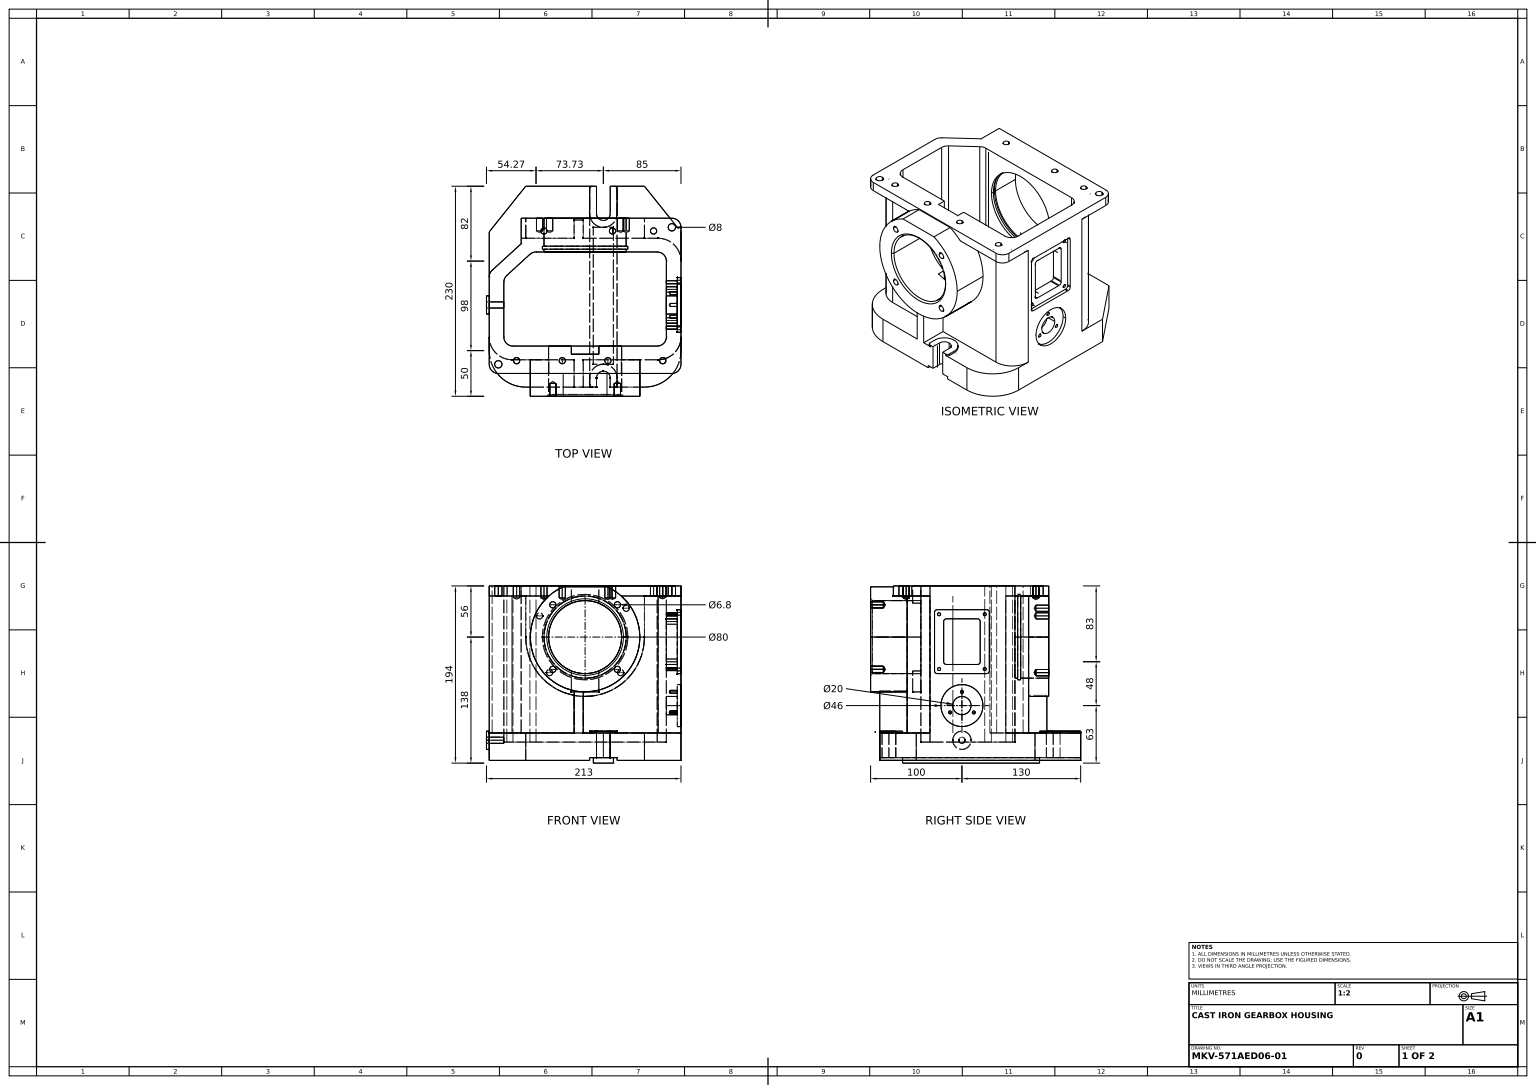
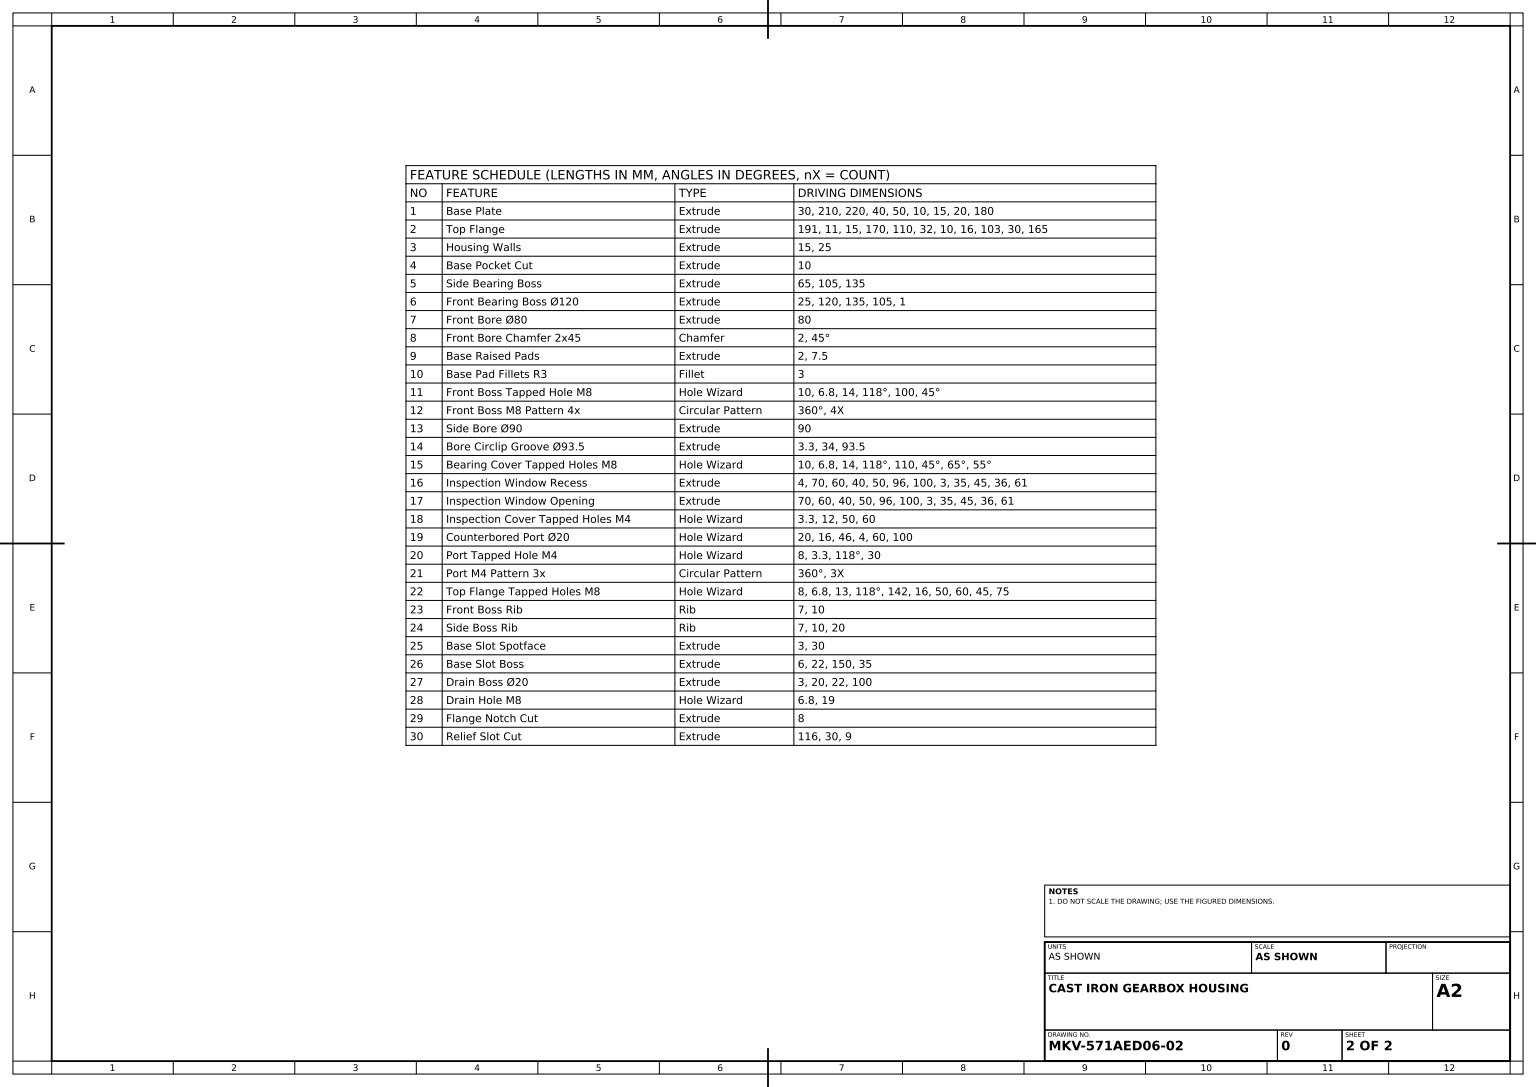
from build123d import *

# Parameters (mm, degrees)
BASE_PLATE_DEPTH                       = 30
TOP_FLANGE_DEPTH                       = 11
HOUSING_WALLS_DEPTH                    = 161
BASE_POCKET_CUT_DEPTH                  = 10
SIDE_BEARING_BOSS_REACH                = 287.886
FRONT_BEARING_BOSS_120_REACH           = 318.869
FRONT_BORE_80_REACH                    = 318.869
FRONT_BORE_SKETCH_R                    = 40
FRONT_BORE_CHAMFER_2X45_SIZE           = 2
BASE_RAISED_PADS_DEPTH                 = 2
BASE_PAD_FILLETS_R3_R                  = 3
FRONT_BOSS_M8_PATTERN_4X_COUNT         = 4
SIDE_BORE_90_REACH                     = 294.457
SIDE_BORE_SKETCH_R                     = 45
BORE_START                             = -34
CIRCLIP_GROOVE_SKETCH_R                = 46.75
BORE_CIRCLIP_GROOVE_93_5_DEPTH         = 3.3
BEARING_COVER_TAPPED_HOLES_M8_D        = 6.8
BEARING_COVER_TAPPED_HOLES_M8_DEPTH    = 14
BEARING_COVER_TAPPED_HOLES_M8_TIP      = 2.042926105
INSPECTION_WINDOW_RECESS_DEPTH         = 4
INSPECTION_WINDOW_OPENING_REACH        = 361.139
INSPECTION_COVER_TAPPED_HOLES_M4_D     = 3.3
INSPECTION_COVER_TAPPED_HOLES_M4_DEPTH = 12
COUNTERBORED_PORT_20_D                 = 20
COUNTERBORED_PORT_20_DEPTH             = 16
COUNTERBORED_PORT_20_CBORE_D           = 46
COUNTERBORED_PORT_20_CBORE_DEPTH       = 4
PORT_M4_PATTERN_3X_COUNT               = 3
TOP_FLANGE_TAPPED_HOLES_M8_D           = 6.8
TOP_FLANGE_TAPPED_HOLES_M8_DEPTH       = 13
TOP_FLANGE_TAPPED_HOLES_M8_TIP         = 2.042926105
FRONT_BOSS_RIB_REACH                   = 314.13
FRONT_BOSS_RIB_SKETCH_WALL_W           = 671.259561472
FRONT_BOSS_RIB_SKETCH_WALL_H           = 10
SIDE_BOSS_RIB_REACH                    = 314.13
SIDE_BOSS_RIB_SKETCH_WALL_W            = 666.259561472
SIDE_BOSS_RIB_SKETCH_WALL_H            = 10
BASE_SLOT_SPOTFACE_SKETCH_W            = 30
BASE_SLOT_SPOTFACE_SKETCH_H            = 220
BASE_SLOT_SPOTFACE_DEPTH               = 3
BASE_SLOT_BOSS_SKETCH_W                = 22
BASE_SLOT_BOSS_SKETCH_H                = 150
BASE_SLOT_BOSS_DEPTH                   = 6
DRAIN_BOSS_SKETCH_R                    = 10
DRAIN_BOSS_20_DEPTH                    = 3
DRAIN_HOLE_M8_D                        = 6.8
DRAIN_HOLE_M8_DEPTH                    = 19
FLANGE_NOTCH_CUT_REACH                 = 314.57
FLANGE_NOTCH_SKETCH_R                  = 4
RELIEF_SLOT_SKETCH_W                   = 30
RELIEF_SLOT_SKETCH_H                   = 9
RELIEF_SLOT_CUT_DEPTH                  = 116


with BuildPart() as part:
    # Base Plate Sketch → Base Plate (new body)
    with BuildSketch(Plane(origin=(0, 0, 0), x_dir=(1, 0, 0), z_dir=(0, 1, 0))):
        with BuildLine():
            Line((-65, 220), (-105, 170))
            Line((-105, 170), (-105, 40))
            ThreePointArc((-105, 40), (-93.284271247, 11.715728753), (-65, 0))
            Line((-65, 0), (12.5, 0))
            Line((12.5, 0), (12.5, 10))
            ThreePointArc((12.5, 10), (20, 17.5), (27.5, 10))
            Line((27.5, 10), (27.5, 0))
            Line((27.5, 0), (65, 0))
            ThreePointArc((65, 0), (93.284271247, 11.715728753), (105, 40))
            Line((105, 40), (105, 170))
            Line((105, 170), (65, 220))
            Line((65, 220), (27.5, 220))
            Line((27.5, 220), (27.5, 190))
            ThreePointArc((27.5, 190), (20, 182.5), (12.5, 190))
            Line((12.5, 190), (12.5, 220))
            Line((12.5, 220), (-65, 220))
        make_face()
    extrude(amount=BASE_PLATE_DEPTH)



with BuildPart() as body_2:
    # Top Flange Sketch → Top Flange (new body)
    with BuildSketch(Plane(origin=(0, 191, 0), x_dir=(1, 0, 0), z_dir=(0, 1, 0))):
        with BuildLine():
            Line((-95, 15), (95, 15))
            ThreePointArc((95, 15), (102.071067812, 17.928932188), (105, 25))
            Line((105, 25), (105, 175))
            ThreePointArc((105, 175), (102.071067812, 182.071067812), (95, 185))
            Line((95, 185), (-70, 185))
            Line((-70, 185), (-70, 157))
            Line((-70, 157), (-101.747691995, 127.973538747))
            ThreePointArc((-101.747691995, 127.973538747), (-104.150872088, 124.625810611), (-105, 120.593250627))
            Line((-105, 120.593250627), (-105, 25))
            ThreePointArc((-105, 25), (-102.071067812, 17.928932188), (-95, 15))
        make_face()
        with BuildLine():
            Line((-79, 45), (79, 45))
            ThreePointArc((79, 45), (86.071067812, 47.928932188), (89, 55))
            Line((89, 55), (89, 138))
            ThreePointArc((89, 138), (86.071067812, 145.071067812), (79, 148))
            Line((79, 148), (-53.731544683, 148))
            ThreePointArc((-53.731544683, 148), (-57.350737881, 147.322094218), (-60.479236679, 145.38028812))
            Line((-60.479236679, 145.38028812), (-85.747691995, 122.277700402))
            ThreePointArc((-85.747691995, 122.277700402), (-88.150872088, 118.929972266), (-89, 114.897412282))
            Line((-89, 114.897412282), (-89, 55))
            ThreePointArc((-89, 55), (-86.071067812, 47.928932188), (-79, 45))
        make_face(mode=Mode.SUBTRACT)
    extrude(amount=-TOP_FLANGE_DEPTH)


with BuildPart() as part_1:
    add(part.part)

    add(body_2.part)  # Housing Walls merges body 2
    # Housing Walls Sketch → Housing Walls (add)
    with BuildSketch(Plane(origin=(0, 191, 0), x_dir=(1, 0, 0), z_dir=(0, 1, 0))):
        with BuildLine():
            Line((80, 163), (-70, 163))
            Line((-70, 163), (-70, 157))
            Line((-70, 157), (-101.747691995, 127.973538747))
            ThreePointArc((-101.747691995, 127.973538747), (-104.150872088, 124.625810611), (-105, 120.593250627))
            Line((-105, 120.593250627), (-105, 55))
            ThreePointArc((-105, 55), (-97.67766953, 37.32233047), (-80, 30))
            Line((-80, 30), (80, 30))
            ThreePointArc((80, 30), (97.67766953, 37.32233047), (105, 55))
            Line((105, 55), (105, 138))
            ThreePointArc((105, 138), (97.67766953, 155.67766953), (80, 163))
        make_face()
        with BuildLine():
            Line((-60.479236679, 145.38028812), (-85.747691995, 122.277700402))
            ThreePointArc((-85.747691995, 122.277700402), (-88.150872088, 118.929972266), (-89, 114.897412282))
            Line((-89, 114.897412282), (-89, 55))
            ThreePointArc((-89, 55), (-86.071067812, 47.928932188), (-79, 45))
            Line((-79, 45), (79, 45))
            ThreePointArc((79, 45), (86.071067812, 47.928932188), (89, 55))
            Line((89, 55), (89, 138))
            ThreePointArc((89, 138), (86.071067812, 145.071067812), (79, 148))
            Line((79, 148), (-53.731544683, 148))
            ThreePointArc((-53.731544683, 148), (-57.350737881, 147.322094218), (-60.479236679, 145.38028812))
        make_face(mode=Mode.SUBTRACT)
    extrude(amount=-HOUSING_WALLS_DEPTH)

    # Base Pocket Sketch → Base Pocket Cut (cut)
    with BuildSketch(Plane(origin=(0, 30, 0), x_dir=(1, 0, 0), z_dir=(0, 1, 0))):
        with BuildLine():
            Line((-60.479236679, 145.38028812), (-85.747691995, 122.277700402))
            ThreePointArc((-85.747691995, 122.277700402), (-88.150872088, 118.929972266), (-89, 114.897412282))
            Line((-89, 114.897412282), (-89, 55))
            ThreePointArc((-89, 55), (-86.071067812, 47.928932188), (-79, 45))
            Line((-79, 45), (79, 45))
            ThreePointArc((79, 45), (86.071067812, 47.928932188), (89, 55))
            Line((89, 55), (89, 138))
            ThreePointArc((89, 138), (86.071067812, 145.071067812), (79, 148))
            Line((79, 148), (-53.731544683, 148))
            ThreePointArc((-53.731544683, 148), (-57.350737881, 147.322094218), (-60.479236679, 145.38028812))
        make_face()
    extrude(amount=-BASE_POCKET_CUT_DEPTH, mode=Mode.SUBTRACT)

    # Side Bearing Boss Sketch → Side Bearing Boss (add, up to next)
    with BuildSketch(Plane(origin=(0, 0, -185), x_dir=(-1, 0, 0), z_dir=(0, 0, -1)), mode=Mode.PRIVATE) as side_bearing_boss_sk1:
        with BuildLine():
            Line((65, 180), (-65, 180))
            Line((-65, 180), (-65, 135))
            ThreePointArc((-65, 135), (0, 70), (65, 135))
            Line((65, 135), (65, 180))
        make_face()
    side_bearing_boss_tool1 = extrude(side_bearing_boss_sk1.sketch, amount=-SIDE_BEARING_BOSS_REACH, mode=Mode.PRIVATE) - part_1.part
    add(side_bearing_boss_tool1.solids().sort_by_distance((0, 130.87892, -185))[0])

    # Front Bearing Boss Sketch → Front Bearing Boss _120 (add, up to next)
    with BuildSketch(Plane.XY.offset(10), mode=Mode.PRIVATE) as front_bearing_boss_120_sk1:
        with BuildLine():
            Line((-23.979157617, 190), (23.979157617, 190))
            ThreePointArc((23.979157617, 190), (0, 75), (-23.979157617, 190))
        make_face()
    front_bearing_boss_120_tool1 = extrude(front_bearing_boss_120_sk1.sketch, amount=-FRONT_BEARING_BOSS_120_REACH, mode=Mode.PRIVATE) - part_1.part
    add(front_bearing_boss_120_tool1.solids().sort_by_distance((0, 134.175493, 10))[0])

    # Front Bore Sketch → Front Bore _80 (cut, up to next)
    with BuildSketch(Plane.XY.offset(10), mode=Mode.PRIVATE) as front_bore_80_sk1:
        with Locations((0, 135)):
            Circle(FRONT_BORE_SKETCH_R)
    front_bore_80_tool1 = extrude(front_bore_80_sk1.sketch, amount=-FRONT_BORE_80_REACH, mode=Mode.PRIVATE) & part_1.part
    add(front_bore_80_tool1.solids().sort_by_distance((0, 135, 10))[0], mode=Mode.SUBTRACT)

    # Front Bore Chamfer 2x45
    front_bore_chamfer_2x45_edges = [part_1.edges().sort_by_distance(p)[0] for p in [
        (-40, 135, 10),
    ]]
    chamfer(front_bore_chamfer_2x45_edges, length=FRONT_BORE_CHAMFER_2X45_SIZE)

    # Base Pads Sketch → Base Raised Pads (add)
    with BuildSketch(Plane(origin=(0, 30, 0), x_dir=(1, 0, 0), z_dir=(0, 1, 0))):
        with BuildLine():
            Line((12.5, 220), (12.5, 190))
            ThreePointArc((12.5, 190), (20, 182.5), (27.5, 190))
            Line((27.5, 190), (27.5, 220))
            Line((27.5, 220), (35, 220))
            Line((35, 220), (35, 190))
            ThreePointArc((35, 190), (20, 175), (5, 190))
            Line((5, 190), (5, 220))
            Line((5, 220), (12.5, 220))
        make_face()
        with BuildLine():
            Line((12.5, 0), (12.5, 10))
            ThreePointArc((12.5, 10), (20, 17.5), (27.5, 10))
            Line((27.5, 10), (27.5, 0))
            Line((27.5, 0), (35, 0))
            Line((35, 0), (35, 10))
            ThreePointArc((35, 10), (20, 25), (5, 10))
            Line((5, 10), (5, 0))
            Line((5, 0), (12.5, 0))
        make_face()
    extrude(amount=BASE_RAISED_PADS_DEPTH)

    # Base Pad Fillets R3
    base_pad_fillets_r3_edges = [part_1.edges().sort_by_distance(p)[0] for p in [
        (5, 31, -220),
        (35, 31, -220),
        (5, 31, 0),
        (35, 31, 0),
    ]]
    fillet(base_pad_fillets_r3_edges, radius=BASE_PAD_FILLETS_R3_R)

    # Sketch10 → Front Boss Tapped Hole M8 (revolve, cut)
    with BuildSketch(Plane(origin=(35.355339059, 170.355339059, 10), x_dir=(0, -1, 0), z_dir=(1, 0, 0))):
        Polygon((0, 0), (0, 16.042926105), (3.4, 14), (3.4, 0), align=None)
    front_boss_tapped_hole_m8 = revolve(axis=Axis((35.355339059, 170.355339059, 16.35), (0, 0, -1)), mode=Mode.SUBTRACT)

    # Front Boss M8 Pattern 4x: Front Boss Tapped Hole M8 ×4 about axis
    front_boss_m8_pattern_4x_axis = Axis((0, 135, 0), (0, 0, 1))
    for i in range(1, FRONT_BOSS_M8_PATTERN_4X_COUNT):
        add(front_boss_tapped_hole_m8.rotate(front_boss_m8_pattern_4x_axis, i * 360 / FRONT_BOSS_M8_PATTERN_4X_COUNT), mode=Mode.SUBTRACT)

    # Side Bore Sketch → Side Bore _90 (cut, up to next)
    with BuildSketch(Plane(origin=(0, 0, -185), x_dir=(-1, 0, 0), z_dir=(0, 0, -1)), mode=Mode.PRIVATE) as side_bore_90_sk1:
        with Locations((0, 135)):
            Circle(SIDE_BORE_SKETCH_R)
    side_bore_90_tool1 = extrude(side_bore_90_sk1.sketch, amount=-SIDE_BORE_90_REACH, mode=Mode.PRIVATE) & part_1.part
    add(side_bore_90_tool1.solids().sort_by_distance((0, 135, -185))[0], mode=Mode.SUBTRACT)

    # Circlip Groove Sketch → Bore Circlip Groove _93.5 (cut)
    with BuildSketch(Plane(origin=(0, 0, -185), x_dir=(-1, 0, 0), z_dir=(0, 0, -1)).offset(BORE_START)):
        with Locations((0, 135)):
            Circle(CIRCLIP_GROOVE_SKETCH_R)
    extrude(amount=BORE_CIRCLIP_GROOVE_93_5_DEPTH, mode=Mode.SUBTRACT)

    # Bearing Cover Tapped Holes M8
    with Locations(Plane(origin=(0, 0, -185), x_dir=(-1, 0, 0), z_dir=(0, 0, -1))):
        with Locations((38.890872965, 96.109127035), (-38.890872965, 96.109127035), (-45.053362436, 166.546703999), (49.846928287, 158.244004396)):
            Hole(BEARING_COVER_TAPPED_HOLES_M8_D / 2, depth=BEARING_COVER_TAPPED_HOLES_M8_DEPTH)
            with Locations((0, 0, -(BEARING_COVER_TAPPED_HOLES_M8_DEPTH + BEARING_COVER_TAPPED_HOLES_M8_TIP / 2))):  # 118° drill point
                Cone(0, BEARING_COVER_TAPPED_HOLES_M8_D / 2, BEARING_COVER_TAPPED_HOLES_M8_TIP, mode=Mode.SUBTRACT)

    # Inspection Window Sketch → Inspection Window Recess (cut)
    with BuildSketch(Plane(origin=(105, 0, 0), x_dir=(0, 0, -1), z_dir=(1, 0, 0))):
        with BuildLine():
            ThreePointArc((63, 95), (60.878679656, 95.878679656), (60, 98))
            Line((60, 98), (60, 162))
            ThreePointArc((60, 162), (60.878679656, 164.121320344), (63, 165))
            Line((63, 165), (117, 165))
            ThreePointArc((117, 165), (119.121320344, 164.121320344), (120, 162))
            Line((120, 162), (120, 98))
            ThreePointArc((120, 98), (119.121320344, 95.878679656), (117, 95))
            Line((117, 95), (63, 95))
        make_face()
        with BuildLine():
            Line((73, 105), (107, 105))
            ThreePointArc((107, 105), (109.121320344, 105.878679656), (110, 108))
            Line((110, 108), (110, 152))
            ThreePointArc((110, 152), (109.121320344, 154.121320344), (107, 155))
            Line((107, 155), (73, 155))
            ThreePointArc((73, 155), (70.878679656, 154.121320344), (70, 152))
            Line((70, 152), (70, 108))
            ThreePointArc((70, 108), (70.878679656, 105.878679656), (73, 105))
        make_face(mode=Mode.SUBTRACT)
    extrude(amount=-INSPECTION_WINDOW_RECESS_DEPTH, mode=Mode.SUBTRACT)

    # Sketch16_3 → Inspection Window Opening (cut, up to next)
    with BuildSketch(Plane(origin=(105, 0, 0), x_dir=(0, 0, -1), z_dir=(1, 0, 0)), mode=Mode.PRIVATE) as inspection_window_opening_sk1:
        with BuildLine():
            ThreePointArc((73, 105), (70.878679656, 105.878679656), (70, 108))
            Line((70, 108), (70, 152))
            ThreePointArc((70, 152), (70.878679656, 154.121320344), (73, 155))
            Line((73, 155), (107, 155))
            ThreePointArc((107, 155), (109.121320344, 154.121320344), (110, 152))
            Line((110, 152), (110, 108))
            ThreePointArc((110, 108), (109.121320344, 105.878679656), (107, 105))
            Line((107, 105), (73, 105))
        make_face()
    inspection_window_opening_tool1 = extrude(inspection_window_opening_sk1.sketch, amount=-INSPECTION_WINDOW_OPENING_REACH, mode=Mode.PRIVATE) & part_1.part
    add(inspection_window_opening_tool1.solids().sort_by_distance((105, 130, -90))[0], mode=Mode.SUBTRACT)

    # Inspection Cover Tapped Holes M4
    with Locations(Plane(origin=(101, 0, 0), x_dir=(0, 0, -1), z_dir=(1, 0, 0))):
        with Locations((65, 160), (115, 100), (65, 100), (115, 160)):
            Hole(INSPECTION_COVER_TAPPED_HOLES_M4_D / 2, depth=INSPECTION_COVER_TAPPED_HOLES_M4_DEPTH)

    # Counterbored Port _20
    with Locations(Plane(origin=(105, 0, 0), x_dir=(0, 0, -1), z_dir=(1, 0, 0))):
        with Locations((90, 60)):
            CounterBoreHole(COUNTERBORED_PORT_20_D / 2, COUNTERBORED_PORT_20_CBORE_D / 2, COUNTERBORED_PORT_20_CBORE_DEPTH, depth=COUNTERBORED_PORT_20_DEPTH)

    # Sketch22 → Port Tapped Hole M4 (revolve, cut)
    with BuildSketch(Plane(origin=(101, 75, -90), x_dir=(0, 0, -1), z_dir=(0, 1, 0))):
        Polygon((0, 0), (0, 8.991420021), (1.65, 8), (1.65, 0), align=None)
    port_tapped_hole_m4 = revolve(axis=Axis((107.35, 75, -90), (-1, 0, 0)), mode=Mode.SUBTRACT)

    # Port M4 Pattern 3x: Port Tapped Hole M4 ×3 about axis
    port_m4_pattern_3x_axis = Axis((0, 60, -90), (1, 0, 0))
    for i in range(1, PORT_M4_PATTERN_3X_COUNT):
        add(port_tapped_hole_m4.rotate(port_m4_pattern_3x_axis, i * 360 / PORT_M4_PATTERN_3X_COUNT), mode=Mode.SUBTRACT)

    # Top Flange Tapped Holes M8
    with Locations(Plane(origin=(0, 191, 0), x_dir=(1, 0, 0), z_dir=(0, 1, 0))):
        with Locations((-45, 171), (75, 171), (-75, 29), (85, 29), (-25, 29), (25, 29), (30, 171)):
            Hole(TOP_FLANGE_TAPPED_HOLES_M8_D / 2, depth=TOP_FLANGE_TAPPED_HOLES_M8_DEPTH)
            with Locations((0, 0, -(TOP_FLANGE_TAPPED_HOLES_M8_DEPTH + TOP_FLANGE_TAPPED_HOLES_M8_TIP / 2))):  # 118° drill point
                Cone(0, TOP_FLANGE_TAPPED_HOLES_M8_D / 2, TOP_FLANGE_TAPPED_HOLES_M8_TIP, mode=Mode.SUBTRACT)

    # Front Boss Rib Sketch wall → Front Boss Rib (add, up to next)
    with BuildSketch(Plane(origin=(-7, 52.5, 0), x_dir=(0, 1, 0), z_dir=(0, 0, 1)), mode=Mode.PRIVATE) as front_boss_rib_sk1:
        Rectangle(FRONT_BOSS_RIB_SKETCH_WALL_W, FRONT_BOSS_RIB_SKETCH_WALL_H)
    front_boss_rib_tool1 = extrude(front_boss_rib_sk1.sketch, amount=-FRONT_BOSS_RIB_REACH, mode=Mode.PRIVATE) - part_1.part
    add(front_boss_rib_tool1.solids().sort_by_distance((-7, 52.5, 0))[0])

    # Side Boss Rib Sketch wall → Side Boss Rib (add, up to next)
    with BuildSketch(Plane(origin=(-7, 50, -183), x_dir=(0, -1, 0), z_dir=(0, 0, -1)), mode=Mode.PRIVATE) as side_boss_rib_sk1:
        Rectangle(SIDE_BOSS_RIB_SKETCH_WALL_W, SIDE_BOSS_RIB_SKETCH_WALL_H)
    side_boss_rib_tool1 = extrude(side_boss_rib_sk1.sketch, amount=-SIDE_BOSS_RIB_REACH, mode=Mode.PRIVATE) - part_1.part
    add(side_boss_rib_tool1.solids().sort_by_distance((-7, 50, -183))[0])

    # Base Slot Spotface Sketch → Base Slot Spotface (cut)
    with BuildSketch(Plane.XZ):
        with Locations((20, -110)):
            Rectangle(BASE_SLOT_SPOTFACE_SKETCH_W, BASE_SLOT_SPOTFACE_SKETCH_H)
    extrude(amount=-BASE_SLOT_SPOTFACE_DEPTH, mode=Mode.SUBTRACT)

    # Base Slot Boss Sketch → Base Slot Boss (add)
    with BuildSketch(Plane.XZ.offset(-3)):
        with Locations((20, -100)):
            Rectangle(BASE_SLOT_BOSS_SKETCH_W, BASE_SLOT_BOSS_SKETCH_H)
    extrude(amount=BASE_SLOT_BOSS_DEPTH)

    # Drain Boss Sketch → Drain Boss _20 (add)
    with BuildSketch(Plane.ZY.offset(105)):
        with Locations((-90, 22)):
            Circle(DRAIN_BOSS_SKETCH_R)
    extrude(amount=DRAIN_BOSS_20_DEPTH)

    # Drain Hole M8
    with Locations(Plane.ZY.offset(108)):
        with Locations((-90, 22)):
            Hole(DRAIN_HOLE_M8_D / 2, depth=DRAIN_HOLE_M8_DEPTH)

    # Flange Notch Sketch → Flange Notch Cut (cut, up to next)
    with BuildSketch(Plane(origin=(0, 191, 0), x_dir=(1, 0, 0), z_dir=(0, 1, 0)), mode=Mode.PRIVATE) as flange_notch_cut_sk1:
        with Locations(Location((-95, 25, 0), (0, 0, 270))):
            Circle(FLANGE_NOTCH_SKETCH_R)
    flange_notch_cut_tool1 = extrude(flange_notch_cut_sk1.sketch, amount=-FLANGE_NOTCH_CUT_REACH, mode=Mode.PRIVATE) & part_1.part
    # Flange Notch Sketch → Flange Notch Cut (cut, up to next)
    with BuildSketch(Plane(origin=(0, 191, 0), x_dir=(1, 0, 0), z_dir=(0, 1, 0)), mode=Mode.PRIVATE) as flange_notch_cut_sk2:
        with Locations(Location((95, 175, 0), (0, 0, 270))):
            Circle(FLANGE_NOTCH_SKETCH_R)
    flange_notch_cut_tool2 = extrude(flange_notch_cut_sk2.sketch, amount=-FLANGE_NOTCH_CUT_REACH, mode=Mode.PRIVATE) & part_1.part
    add(flange_notch_cut_tool1.solids().sort_by_distance((-95, 191, -25))[0], mode=Mode.SUBTRACT)
    add(flange_notch_cut_tool2.solids().sort_by_distance((95, 191, -175))[0], mode=Mode.SUBTRACT)

    # Relief Slot Sketch → Relief Slot Cut (cut)
    with BuildSketch(Plane(origin=(0, 191, 0), x_dir=(1, 0, 0), z_dir=(0, 1, 0))):
        with Locations((0, 40.5)):
            Rectangle(RELIEF_SLOT_SKETCH_W, RELIEF_SLOT_SKETCH_H)
    extrude(amount=-RELIEF_SLOT_CUT_DEPTH, mode=Mode.SUBTRACT)


solid = part_1.part
